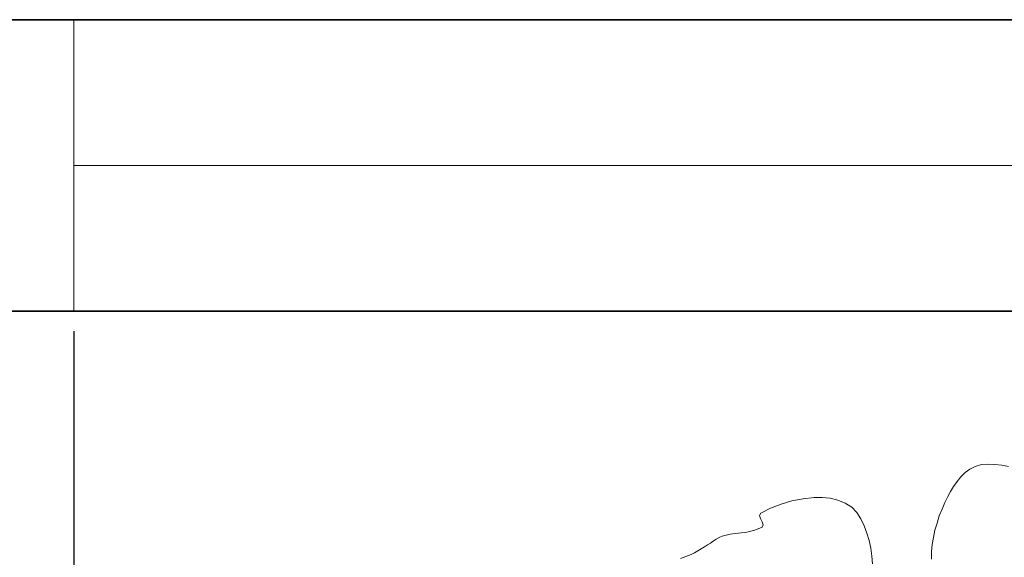
# Model space of a CAD drawing. Units: inches. Extents: x 1484 to 2008, y 1843 to 2590.
# Tile 16 of 21: x 1802 to 1832, y 2201 to 2217. Entities that reach past the tile are written whole.
import ezdxf

# ---------------------------------------------------------------- set-up
doc = ezdxf.new("R2010")
doc.units = ezdxf.units.IN
for name, color, linetype, lineweight in [('A-ANNO-DIMS', 2, 'Continuous', 18), ('A-FURN', 8, 'Continuous', 18), ('A-GLAZ', 4, 'Continuous', 18), ('A-WALL', 7, 'Continuous', 35)]:
    doc.layers.add(name, color=color, linetype=linetype, lineweight=lineweight)
doc.styles.get("Standard").update_dxf_attribs({"font": 'arial.ttf'})
doc.dimstyles.new('ISO-25', dxfattribs={"dimtxt": 7, "dimasz": 2.5, "dimexe": 1.25, "dimexo": 0.625, "dimtad": 1, "dimdec": 0, "dimlunit": 3, "dimtxsty": 'Standard', "dimcen": 2.5, "dimadec": 0, "dimazin": 0, "dimtfac": 1, "dimtdec": 0, "dimtmove": 0, "dimatfit": 3, "dimfxl": 1, "dimarcsym": 0})

# ---------------------------------------------------------------- blocks, each defined once
blk = doc.blocks.new('*D2')
at = {"layer": 'A-ANNO-DIMS', "color": 0, "lineweight": -2, "transparency": 16777216}
for p, q in [((1602.92, 2217.928), (1602.92, 2236.385)), ((1899.92, 2217.928), (1899.92, 2236.385)), ((1605.42, 2235.135), (1897.42, 2235.135))]:
    blk.add_line(p, q, dxfattribs=at)
at = {"layer": 'A-ANNO-DIMS', "color": 0, "transparency": 16777216}
for points in [[(1605.42, 2235.552), (1605.42, 2234.719), (1602.92, 2235.135)], [(1897.42, 2235.552), (1897.42, 2234.719), (1899.92, 2235.135)]]:
    blk.add_solid(points, dxfattribs=at)
at = {"layer": 'Defpoints', "color": 0, "transparency": 16777216}
for p in [(1899.92, 2235.135), (1602.92, 2217.303), (1899.92, 2217.303)]:
    blk.add_point(p, dxfattribs=at)
at = {"layer": 'A-ANNO-DIMS', "color": 0, "transparency": 16777216, "insert": (1750.407, 2239.334), "char_height": 7, "attachment_point": 5}
blk.add_mtext('24\'-9"', dxfattribs=at)
blk = doc.blocks.new('BED-DOUBLE')
for p, q in [((28.429, 84.304), (28.269, 84.221)), ((28.626, 84.36), (28.429, 84.304)), ((28.83, 84.378), (28.626, 84.36)), ((29.039, 84.367), (28.83, 84.378)), ((29.252, 84.339), (29.039, 84.367)), ((29.466, 84.304), (29.252, 84.339)), ((27.993, 83.987), (27.874, 83.843)), ((28.125, 84.114), (27.993, 83.987)), ((28.269, 84.221), (28.125, 84.114)), ((27.767, 83.688), (27.669, 83.525)), ((27.874, 83.843), (27.767, 83.688)), ((23.115, 83.305), (23.459, 83.342)), ((23.459, 83.342), (23.703, 83.345)), ((23.703, 83.345), (23.949, 83.319)), ((27.581, 83.359), (27.5, 83.194)), ((27.669, 83.525), (27.581, 83.359)), ((22.115, 83.013), (22.439, 83.14)), ((22.439, 83.14), (22.774, 83.237)), ((22.774, 83.237), (23.115, 83.305)), ((23.949, 83.319), (24.19, 83.261)), ((24.19, 83.261), (24.417, 83.169)), ((24.417, 83.169), (24.62, 83.041)), ((24.62, 83.041), (24.781, 82.878)), ((27.5, 83.194), (27.408, 82.986)), ((21.775, 82.793), (21.807, 82.857)), ((21.804, 82.697), (21.775, 82.793)), ((21.807, 82.857), (22.115, 83.013)), ((24.781, 82.878), (24.905, 82.683)), ((27.325, 82.774), (27.253, 82.557)), ((27.408, 82.986), (27.325, 82.774)), ((21.622, 82.331), (21.85, 82.43)), ((21.852, 82.592), (21.804, 82.697)), ((21.85, 82.43), (21.881, 82.496)), ((21.881, 82.496), (21.852, 82.592)), ((24.905, 82.683), (25.002, 82.466)), ((25.002, 82.466), (25.082, 82.24)), ((27.253, 82.557), (27.191, 82.337)), ((20.432, 82.058), (20.524, 82.112)), ((20.524, 82.112), (20.621, 82.153)), ((20.621, 82.153), (20.867, 82.211)), ((20.867, 82.211), (21.122, 82.245)), ((21.122, 82.245), (21.376, 82.277)), ((21.376, 82.277), (21.622, 82.331)), ((25.082, 82.24), (25.156, 82.016)), ((27.142, 82.113), (27.107, 81.889)), ((27.191, 82.337), (27.142, 82.113)), ((19.968, 81.755), (20.067, 81.817)), ((20.067, 81.817), (20.166, 81.878)), ((20.166, 81.878), (20.256, 81.936)), ((20.256, 81.936), (20.344, 81.998)), ((20.344, 81.998), (20.432, 82.058)), ((25.156, 82.016), (25.212, 81.78)), ((27.107, 81.889), (27.086, 81.663)), ((19.333, 81.457), (19.499, 81.518)), ((19.499, 81.518), (19.662, 81.586)), ((19.662, 81.586), (19.767, 81.637)), ((19.767, 81.637), (19.868, 81.694)), ((19.868, 81.694), (19.968, 81.755)), ((25.212, 81.78), (25.241, 81.536)), ((25.241, 81.536), (25.262, 81.291)), ((27.086, 81.663), (27.081, 81.437))]:
    blk.add_line(p, q)
blk = doc.blocks.new('WIN-60IN')
for p, q in [((0, 4.5), (0, -4.5)), ((0, -4.5), (0, 0)), ((0, 0), (60, 0))]:
    blk.add_line(p, q)
blk = doc.blocks.new('*D13')
at = {"layer": 'A-ANNO-DIMS', "color": 0, "lineweight": -2, "transparency": 16777216}
for p, q in [((1803.22, 2207.678), (1803.22, 2198.053)), ((1863.22, 2207.678), (1863.22, 2198.053)), ((1805.72, 2199.303), (1860.72, 2199.303)), ((1863.22, 2199.303), (2008.197, 2199.303))]:
    blk.add_line(p, q, dxfattribs=at)
at = {"layer": 'A-ANNO-DIMS', "color": 0, "transparency": 16777216}
for points in [[(1805.72, 2199.72), (1805.72, 2198.886), (1803.22, 2199.303)], [(1860.72, 2199.72), (1860.72, 2198.886), (1863.22, 2199.303)]]:
    blk.add_solid(points, dxfattribs=at)
at = {"layer": 'Defpoints', "color": 0, "transparency": 16777216}
for p in [(1803.22, 2208.303), (1863.22, 2208.303), (1863.22, 2199.303)]:
    blk.add_point(p, dxfattribs=at)
at = {"layer": 'A-ANNO-DIMS', "color": 0, "transparency": 16777216, "insert": (1936.959, 2203.55), "char_height": 7, "attachment_point": 5}
blk.add_mtext('BEDROOM WINDOW 5\'-0" TYP.', dxfattribs=at)

msp = doc.modelspace()

# ---------------------------------------------------------------- linework, layer by layer
at = {"layer": 'A-WALL'}
for p, q in [((1602.92, 2217.303), (1899.92, 2217.303)), ((1602.92, 2217.303), (1899.92, 2217.303)), ((1758.92, 2208.303), (1890.92, 2208.303))]:
    msp.add_line(p, q, dxfattribs=at)

# ---------------------------------------------------------------- block references
at = {"layer": 'A-FURN'}
msp.add_blockref('BED-DOUBLE', (1802.632, 2119.201), dxfattribs=at)
at = {"layer": 'A-GLAZ'}
msp.add_blockref('WIN-60IN', (1803.22, 2212.803), dxfattribs=at)

# ---------------------------------------------------------------- dimensions: what is measured, and where the dimension line sits
at = {"layer": 'A-ANNO-DIMS'}
dim = msp.add_linear_dim(base=(1899.92, 2235.135), p1=(1602.92, 2217.303), p2=(1899.92, 2217.303), dimstyle='ISO-25', override={"dimclrd": 0, "dimclre": 0, "dimclrt": 0}, dxfattribs=at)
dim.commit()
dim.dimension.update_dxf_attribs({"geometry": '*D2', "text_midpoint": (1750.407, 2235.135), "dimtype": 160})
dim = msp.add_linear_dim(base=(1863.22, 2199.303), p1=(1803.22, 2208.303), p2=(1863.22, 2208.303), text='BEDROOM WINDOW <> TYP.', dimstyle='ISO-25', override={"dimdec": 1, "dimlfac": 1, "dimrnd": 0, "dimzin": 1, "dimdsep": 46, "dimlunit": 4, "dimfrac": 2}, dxfattribs=at)
dim.commit()
dim.dimension.update_dxf_attribs({"geometry": '*D13', "text_midpoint": (1936.959, 2203.55)})

doc.saveas('drawing.dxf')
